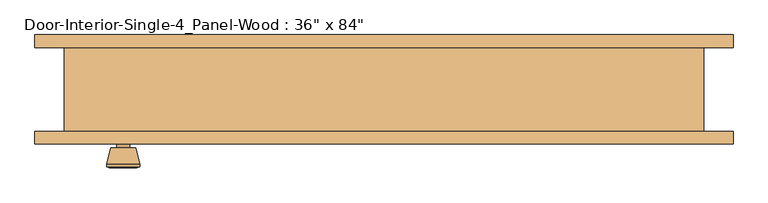
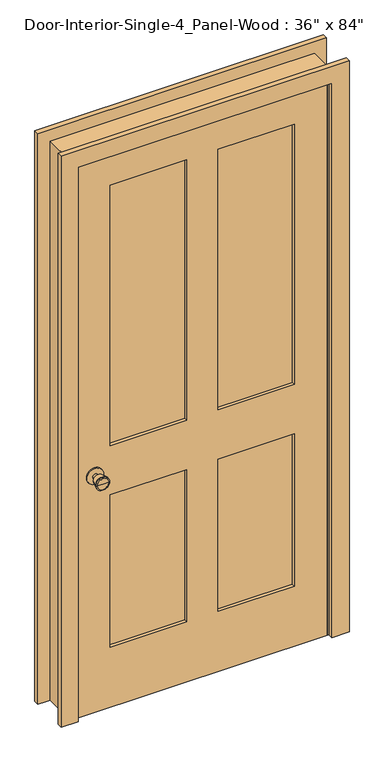
"""IFC4 building model written with IfcOpenShell, lengths in millimetres: door geometry."""

from ifc_helpers import new_model, si_unit, point, frame, frame_2d, origin, place, context, project, spatial, polyline, circle_curve, trimmed, segment, composite_curve, outline, extrude, faceted_brep, source, transform, mapped, element, save
from ifc_brep_helpers import plane_surface, cylinder_surface, revolved_surface, advanced_brep


def door_a823658d(model_context):
    return source(origin(), model_context, "Body", "SolidModel", [
        advanced_brep(
        [(-393.7, -19.4, 914.4), (-403.7, -19.4, 914.4), (-383.7, -19.4, 914.4), (-373.2241324, 29.6, 914.4), (-414.1758676, 29.6, 914.4), (-393.7, 29.6, 914.4), (-368.7, 27.7721319, 914.4), (-418.7, 27.7721319, 914.4), (-368.7, 24.3084537, 914.4), (-418.7, 24.3084537, 914.4), (-375.063764, -0.4, 914.4), (-412.336236, -0.4, 914.4), (-383.7, -0.4, 914.4), (-403.7, -0.4, 914.4)],
        [
            (0, 1),
            (1, 2, circle_curve(frame((-393.7, -19.4, 914.4), z_axis=(0.0, -1.0, 0.0), x_axis=(-1.0, 0.0, 0.0)), 10.0)),
            (2, 0),
            (2, 1, circle_curve(frame((-393.7, -19.4, 914.4), z_axis=(0.0, -1.0, 0.0), x_axis=(-1.0, 0.0, 0.0)), 10.0)),
            (3, 4, circle_curve(frame((-393.7, 29.6, 914.4), z_axis=(0.0, 1.0, 0.0), x_axis=(-1.0, 0.0, 0.0)), 20.4758676)),
            (4, 5),
            (5, 3),
            (4, 3, circle_curve(frame((-393.7, 29.6, 914.4), z_axis=(0.0, 1.0, 0.0), x_axis=(-1.0, 0.0, 0.0)), 20.4758676)),
            (6, 7, circle_curve(frame((-393.7, 27.7721319, 914.4), z_axis=(0.0, 1.0, 0.0), x_axis=(-1.0, 0.0, 0.0)), 25.0)),
            (7, 4),
            (3, 6),
            (7, 6, circle_curve(frame((-393.7, 27.7721319, 914.4), z_axis=(0.0, 1.0, 0.0), x_axis=(-1.0, 0.0, 0.0)), 25.0)),
            (8, 9, circle_curve(frame((-393.7, 24.3084537, 914.4), z_axis=(0.0, 1.0, 0.0), x_axis=(-1.0, 0.0, 0.0)), 25.0)),
            (9, 7),
            (6, 8),
            (9, 8, circle_curve(frame((-393.7, 24.3084537, 914.4), z_axis=(0.0, 1.0, 0.0), x_axis=(-1.0, 0.0, 0.0)), 25.0)),
            (10, 11, circle_curve(frame((-393.7, -0.4, 914.4), z_axis=(0.0, 1.0, 0.0), x_axis=(-1.0, 0.0, 0.0)), 18.636236)),
            (11, 9),
            (8, 10),
            (11, 10, circle_curve(frame((-393.7, -0.4, 914.4), z_axis=(0.0, 1.0, 0.0), x_axis=(-1.0, 0.0, 0.0)), 18.636236)),
            (12, 13, circle_curve(frame((-393.7, -0.4, 914.4), z_axis=(0.0, 1.0, 0.0), x_axis=(-1.0, 0.0, 0.0)), 10.0)),
            (13, 11),
            (10, 12),
            (13, 12, circle_curve(frame((-393.7, -0.4, 914.4), z_axis=(0.0, 1.0, 0.0), x_axis=(-1.0, 0.0, 0.0)), 10.0)),
            (1, 13),
            (12, 2),
        ],
        [
            plane_surface(frame((-393.7, -19.4, 914.4), z_axis=(0.0, -1.0, 0.0), x_axis=(-1.0, 0.0, 0.0))),
            plane_surface(frame((-393.7, 29.6, 914.4), z_axis=(0.0, 1.0, 0.0), x_axis=(-1.0, 0.0, 0.0))),
            revolved_surface(polyline([(-414.1758676, 29.6, 914.4), (-418.7, 27.7721319, 914.4)]), (-393.7, -19.4, 914.4), (0.0, -1.0, 0.0)),
            cylinder_surface(frame((-393.7, -19.4, 914.4), z_axis=(0.0, -1.0, 0.0), x_axis=(-1.0, 0.0, 0.0)), 25.0),
            revolved_surface(polyline([(-418.7, 24.3084537, 914.4), (-412.336236, -0.4, 914.4)]), (-393.7, -19.4, 914.4), (0.0, -1.0, 0.0)),
            plane_surface(frame((-393.7, -0.4, 914.4), z_axis=(0.0, -1.0, 0.0), x_axis=(-1.0, 0.0, 0.0))),
            cylinder_surface(frame((-393.7, -19.4, 914.4), z_axis=(0.0, -1.0, 0.0), x_axis=(-1.0, 0.0, 0.0)), 10.0),
        ],
        [
            (0, [[1, 2, 3]]),
            (0, [[-3, 4, -1]]),
            (1, [[5, 6, 7]]),
            (1, [[8, -7, -6]]),
            (2, [[9, 10, -5, 11]]),
            (2, [[12, -11, -8, -10]]),
            (3, [[13, 14, -9, 15]]),
            (3, [[16, -15, -12, -14]]),
            (4, [[17, 18, -13, 19]]),
            (4, [[20, -19, -16, -18]]),
            (5, [[21, 22, -17, 23]]),
            (5, [[24, -23, -20, -22]]),
            (6, [[-2, 25, -21, 26]]),
            (6, [[-4, -26, -24, -25]]),
        ],
    ),
        extrude(outline(composite_curve([segment(trimmed(circle_curve(frame_2d((914.4, -393.7)), 30.0), [point((914.4, -423.7))], [point((914.4, -363.7))], False, "CARTESIAN"), True, "CONTINUOUS"), segment(trimmed(circle_curve(frame_2d((914.4, -393.7)), 30.0), [point((914.4, -363.7))], [point((914.4, -423.7))], False, "CARTESIAN"), True, "CONTINUOUS")], self_intersect=False)), frame((0.0, -25.4, 0.0), z_axis=(0.0, 1.0, 0.0), x_axis=(0.0, 0.0, 1.0)), (0.0, 0.0, 1.0), 6.0),
        advanced_brep(
        [(-393.7, -66.325, 914.4), (-383.7, -66.325, 914.4), (-403.7, -66.325, 914.4), (-373.2241324, -115.325, 914.4), (-393.7, -115.325, 914.4), (-414.1758676, -115.325, 914.4), (-368.7, -113.4971319, 914.4), (-418.7, -113.4971319, 914.4), (-368.7, -110.0334537, 914.4), (-418.7, -110.0334537, 914.4), (-375.063764, -85.325, 914.4), (-412.336236, -85.325, 914.4), (-383.7, -85.325, 914.4), (-403.7, -85.325, 914.4)],
        [
            (0, 1),
            (1, 2, circle_curve(frame((-393.7, -66.325, 914.4), z_axis=(0.0, 1.0, 0.0), x_axis=(-1.0, 0.0, 0.0)), 10.0)),
            (2, 0),
            (2, 1, circle_curve(frame((-393.7, -66.325, 914.4), z_axis=(0.0, 1.0, 0.0), x_axis=(-1.0, 0.0, 0.0)), 10.0)),
            (3, 4),
            (4, 5),
            (5, 3, circle_curve(frame((-393.7, -115.325, 914.4), z_axis=(0.0, -1.0, 0.0), x_axis=(-1.0, 0.0, 0.0)), 20.4758676)),
            (3, 5, circle_curve(frame((-393.7, -115.325, 914.4), z_axis=(0.0, -1.0, 0.0), x_axis=(-1.0, 0.0, 0.0)), 20.4758676)),
            (6, 3),
            (5, 7),
            (7, 6, circle_curve(frame((-393.7, -113.4971319, 914.4), z_axis=(0.0, -1.0, 0.0), x_axis=(-1.0, 0.0, 0.0)), 25.0)),
            (6, 7, circle_curve(frame((-393.7, -113.4971319, 914.4), z_axis=(0.0, -1.0, 0.0), x_axis=(-1.0, 0.0, 0.0)), 25.0)),
            (8, 6),
            (7, 9),
            (9, 8, circle_curve(frame((-393.7, -110.0334537, 914.4), z_axis=(0.0, -1.0, 0.0), x_axis=(-1.0, 0.0, 0.0)), 25.0)),
            (8, 9, circle_curve(frame((-393.7, -110.0334537, 914.4), z_axis=(0.0, -1.0, 0.0), x_axis=(-1.0, 0.0, 0.0)), 25.0)),
            (10, 8),
            (9, 11),
            (11, 10, circle_curve(frame((-393.7, -85.325, 914.4), z_axis=(0.0, -1.0, 0.0), x_axis=(-1.0, 0.0, 0.0)), 18.636236)),
            (10, 11, circle_curve(frame((-393.7, -85.325, 914.4), z_axis=(0.0, -1.0, 0.0), x_axis=(-1.0, 0.0, 0.0)), 18.636236)),
            (12, 10),
            (11, 13),
            (13, 12, circle_curve(frame((-393.7, -85.325, 914.4), z_axis=(0.0, -1.0, 0.0), x_axis=(-1.0, 0.0, 0.0)), 10.0)),
            (12, 13, circle_curve(frame((-393.7, -85.325, 914.4), z_axis=(0.0, -1.0, 0.0), x_axis=(-1.0, 0.0, 0.0)), 10.0)),
            (1, 12),
            (13, 2),
        ],
        [
            plane_surface(frame((-393.7, -66.325, 914.4), z_axis=(0.0, 1.0, 0.0), x_axis=(-1.0, 0.0, 0.0))),
            plane_surface(frame((-393.7, -115.325, 914.4), z_axis=(0.0, -1.0, 0.0), x_axis=(-1.0, 0.0, 0.0))),
            revolved_surface(polyline([(-414.1758676, -115.325, 914.4), (-418.7, -113.4971319, 914.4)]), (-393.7, -66.325, 914.4), (0.0, 1.0, 0.0)),
            cylinder_surface(frame((-393.7, -66.325, 914.4), z_axis=(0.0, 1.0, 0.0), x_axis=(-1.0, 0.0, 0.0)), 25.0),
            revolved_surface(polyline([(-418.7, -110.0334537, 914.4), (-412.336236, -85.325, 914.4)]), (-393.7, -66.325, 914.4), (0.0, 1.0, 0.0)),
            plane_surface(frame((-393.7, -85.325, 914.4), z_axis=(0.0, 1.0, 0.0), x_axis=(-1.0, 0.0, 0.0))),
            cylinder_surface(frame((-393.7, -66.325, 914.4), z_axis=(0.0, 1.0, 0.0), x_axis=(-1.0, 0.0, 0.0)), 10.0),
        ],
        [
            (0, [[1, 2, 3]]),
            (0, [[-3, 4, -1]]),
            (1, [[5, 6, 7]]),
            (1, [[-6, -5, 8]]),
            (2, [[9, -7, 10, 11]]),
            (2, [[-10, -8, -9, 12]]),
            (3, [[13, -11, 14, 15]]),
            (3, [[-14, -12, -13, 16]]),
            (4, [[17, -15, 18, 19]]),
            (4, [[-18, -16, -17, 20]]),
            (5, [[21, -19, 22, 23]]),
            (5, [[-22, -20, -21, 24]]),
            (6, [[25, -23, 26, -2]]),
            (6, [[-26, -24, -25, -4]]),
        ],
    ),
        extrude(outline(composite_curve([segment(trimmed(circle_curve(frame_2d((914.4, -393.7)), 30.0), [point((914.4, -423.7))], [point((914.4, -363.7))], False, "CARTESIAN"), True, "CONTINUOUS"), segment(trimmed(circle_curve(frame_2d((914.4, -393.7)), 30.0), [point((914.4, -363.7))], [point((914.4, -423.7))], False, "CARTESIAN"), True, "CONTINUOUS")], self_intersect=False)), frame((0.0, -66.325, 0.0), z_axis=(0.0, 1.0, 0.0), x_axis=(0.0, 0.0, 1.0)), (0.0, 0.0, 1.0), 6.0),
        faceted_brep([(482.6, -60.325, 0.0), (457.2, -60.325, 0.0), (457.2, -25.4, 0.0), (444.5, -25.4, 0.0), (444.5, 9.525, 0.0), (457.2, 9.525, 0.0), (457.2, 66.675, 0.0), (482.6, 66.675, 0.0), (482.6, 66.675, 2159.0), (482.6, -60.325, 2159.0), (457.2, 66.675, 2133.6), (-457.2, 66.675, 2133.6), (-457.2, 66.675, 0.0), (-482.6, 66.675, 0.0), (-482.6, 66.675, 2159.0), (457.2, 9.525, 2133.6), (444.5, 9.525, 2120.9), (-444.5, 9.525, 2120.9), (-444.5, 9.525, 0.0), (-457.2, 9.525, 0.0), (-457.2, 9.525, 2133.6), (444.5, -25.4, 2120.9), (457.2, -25.4, 2133.6), (-457.2, -25.4, 2133.6), (-457.2, -25.4, 0.0), (-444.5, -25.4, 0.0), (-444.5, -25.4, 2120.9), (457.2, -60.325, 2133.6), (-482.6, -60.325, 2159.0), (-482.6, -60.325, 0.0), (-457.2, -60.325, 0.0), (-457.2, -60.325, 2133.6)], [[[0, 1, 2, 3, 4, 5, 6, 7]], [[7, 8, 9, 0]], [[6, 10, 11, 12, 13, 14, 8, 7]], [[5, 15, 10, 6]], [[4, 16, 17, 18, 19, 20, 15, 5]], [[3, 21, 16, 4]], [[2, 22, 23, 24, 25, 26, 21, 3]], [[1, 27, 22, 2]], [[0, 9, 28, 29, 30, 31, 27, 1]], [[8, 14, 28, 9]], [[15, 20, 11, 10]], [[21, 26, 17, 16]], [[27, 31, 23, 22]], [[29, 13, 12, 19, 18, 25, 24, 30]], [[14, 13, 29, 28]], [[20, 19, 12, 11]], [[26, 25, 18, 17]], [[31, 30, 24, 23]]]),
        extrude(outline(polyline([(2133.6, -457.2), (0.0, -457.2), (0.0, 457.2), (2133.6, 457.2), (2133.6, -457.2)]), holes=[polyline([(2014.5375, 57.15), (2014.5375, 336.55), (1009.65, 336.55), (1009.65, 57.15), (2014.5375, 57.15)]), polyline([(1009.65, -57.15), (1009.65, -336.55), (2014.5375, -336.55), (2014.5375, -57.15), (1009.65, -57.15)]), polyline([(819.15, 57.15), (819.15, 336.55), (231.775, 336.55), (231.775, 57.15), (819.15, 57.15)]), polyline([(231.775, -57.15), (231.775, -336.55), (819.15, -336.55), (819.15, -57.15), (231.775, -57.15)])]), frame((0.0, -60.325, 0.0), z_axis=(0.0, 1.0, 0.0), x_axis=(0.0, 0.0, 1.0)), (0.0, 0.0, 1.0), 34.925),
        extrude(outline(polyline([(336.55, -37.0416667), (336.55, -48.6833333), (57.15, -48.6833333), (57.15, -37.0416667), (336.55, -37.0416667)])), frame((0.0, 0.0, 1009.65), z_axis=(0.0, 0.0, 1.0), x_axis=(1.0, 0.0, 0.0)), (0.0, 0.0, 1.0), 1004.8875),
        extrude(outline(polyline([(-57.15, -37.0416667), (-57.15, -48.6833333), (-336.55, -48.6833333), (-336.55, -37.0416667), (-57.15, -37.0416667)])), frame((0.0, 0.0, 1009.65), z_axis=(0.0, 0.0, 1.0), x_axis=(1.0, 0.0, 0.0)), (0.0, 0.0, 1.0), 1004.8875),
        extrude(outline(polyline([(336.55, -37.0416667), (336.55, -48.6833333), (57.15, -48.6833333), (57.15, -37.0416667), (336.55, -37.0416667)])), frame((0.0, 0.0, 231.775), z_axis=(0.0, 0.0, 1.0), x_axis=(1.0, 0.0, 0.0)), (0.0, 0.0, 1.0), 587.375),
        extrude(outline(polyline([(-57.15, -37.0416667), (-57.15, -48.6833333), (-336.55, -48.6833333), (-336.55, -37.0416667), (-57.15, -37.0416667)])), frame((0.0, 0.0, 231.775), z_axis=(0.0, 0.0, 1.0), x_axis=(1.0, 0.0, 0.0)), (0.0, 0.0, 1.0), 587.375),
        extrude(outline(polyline([(0.0, 527.05), (2203.45, 527.05), (2203.45, -527.05), (0.0, -527.05), (0.0, -463.55), (2139.95, -463.55), (2139.95, 463.55), (0.0, 463.55), (0.0, 527.05)])), frame((0.0, -79.375, 0.0), z_axis=(0.0, 1.0, 0.0), x_axis=(0.0, 0.0, 1.0)), (0.0, 0.0, 1.0), 19.05),
        extrude(outline(polyline([(0.0, 527.05), (2203.45, 527.05), (2203.45, -527.05), (0.0, -527.05), (0.0, -463.55), (2139.95, -463.55), (2139.95, 463.55), (0.0, 463.55), (0.0, 527.05)])), frame((0.0, 66.675, 0.0), z_axis=(0.0, 1.0, 0.0), x_axis=(0.0, 0.0, 1.0)), (0.0, 0.0, 1.0), 19.05),
    ])


if __name__ == "__main__":
    model = new_model("IFC4")
    model_context = context("Model", 3, world=origin())
    ifc_project = project(units=[si_unit("LENGTHUNIT", "METRE", prefix="MILLI")], contexts=[model_context])
    site = spatial("IfcSite", under=ifc_project)
    building = spatial("IfcBuilding", under=site)
    placement = place(None, origin())
    door_shape = door_a823658d(model_context)
    element("IfcDoor", 1, ObjectType="Door-Interior-Single-4_Panel-Wood : 36\" x 84\"", at=placement, inside=building, context=model_context, shape_type="MappedRepresentation", body=[
        mapped(door_shape, transform((0.0, 0.0, 0.0), x_axis=(1.0, 0.0, 0.0), y_axis=(0.0, 1.0, 0.0), z_axis=(0.0, 0.0, 1.0))),
    ])
    save(model, "model.ifc")

# Revit data of these elements
# Type "Door-Interior-Single-4_Panel-Wood : 36\" x 84\""
#   Type Mark = "10"
#   Assembly Code = "C1020300"
#   Analytic Construction = "Wooden"
#   Top Rail = 0' - 4 11/16"
#   Thickness = 0' - 1 3/8"
#   Thermal Resistance (R) = 2.5876 (h·ft²·°F)/BTU
#   Swing Angle [instance default] = 90.00°
#   Stiles = 0' - 4 3/4"
#   Rough Width = 3' - 2"
#   Rough Height = 7' - 1"
#   Mullion = 0' - 4 1/2"
#   Lock Rail = 0' - 7 1/2"
#   Height = 7' - 0"
#   Width = 3' - 0"
#   Heat Transfer Coefficient (U) = 0.3865 BTU/(h·ft²·°F)
#   Bottom Rail = 0' - 9 1/8"
#   Trim Material = Cherry
#   Panel Material = Cherry
#   Frame Material = Cherry
#   Door Handle Material = Aluminum
#   Visual Light Transmittance = 0
#   Solar Heat Gain Coefficient = 0
#   Wall Closure = (empty or 0)
#   Function = (empty or 0)
# Element 1 (IfcDoor, "Door-Interior-Single-4_Panel-Wood : 36\" x 84\"")
#   Materials on its faces: "Cherry", "Aluminum"
# Materials
#   "Cherry": class "Wood", colour RGB 226 177 128, transparency 0, Description = "Prunus Serotina", Cost = 0
#   "Aluminum": class "Metal", colour RGB 247 247 247, transparency 0, Description = "Aluminum 6061", Cost = 0
